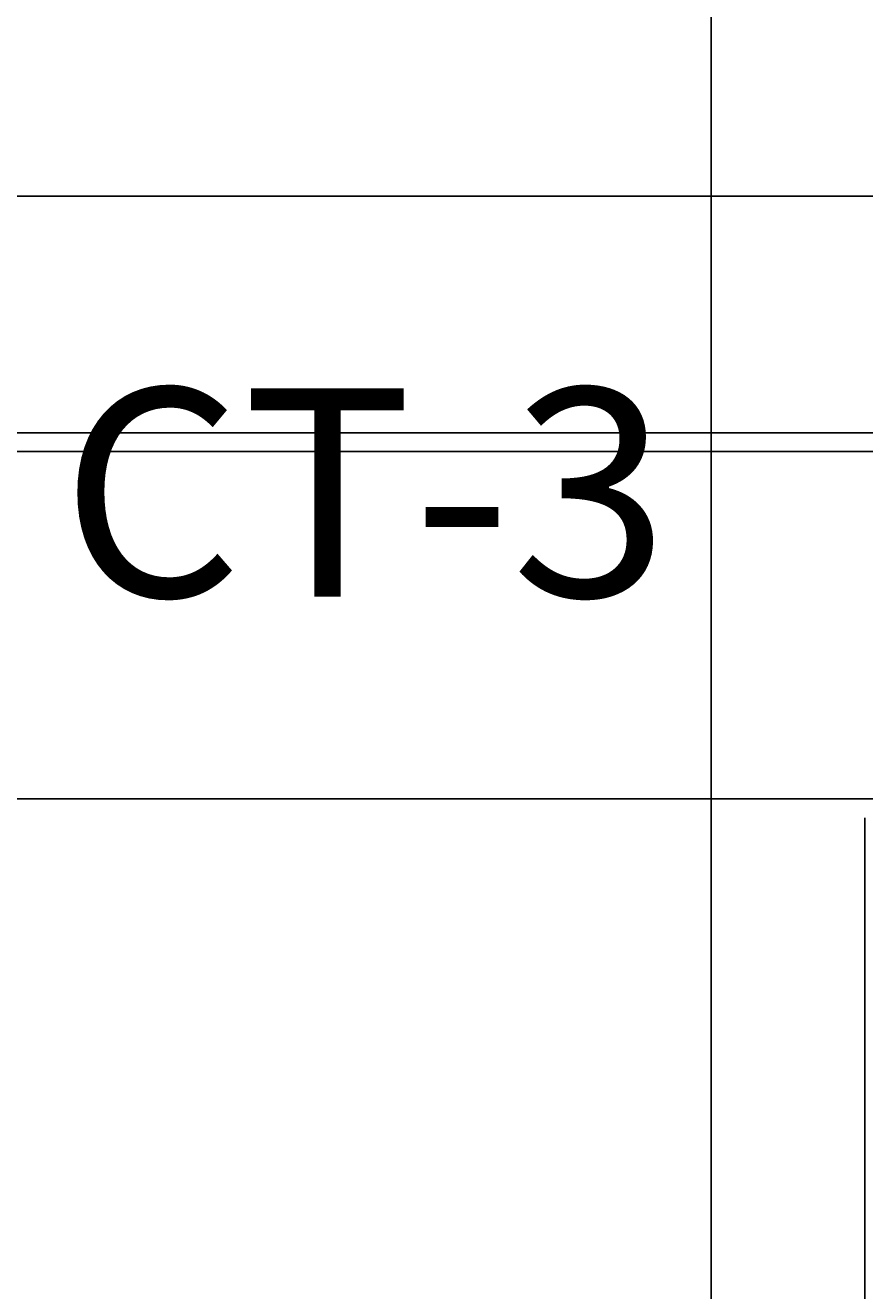
# Model space of a CAD drawing. Units: inches. Extents: x 35362 to 73946, y 43607 to 67532.
# Tile 133 of 134: x 67594 to 68484, y 44948 to 46290. Entities that reach past the tile are written whole.
import ezdxf

# ---------------------------------------------------------------- set-up
doc = ezdxf.new("R2010")
doc.units = ezdxf.units.IN
doc.header["$MEASUREMENT"] = 0
doc.layers.add('A-ANNO-DIMS', color=2, linetype='Continuous', lineweight=18)
doc.layers.add('E-ANNO-TEXT', color=5, linetype='Continuous', lineweight=18)
doc.styles.get("Standard").update_dxf_attribs({"font": 'arial.ttf'})
doc.dimstyles.get("Standard").update_dxf_attribs({"dimtxt": 0.18, "dimasz": 0.18, "dimexe": 0.18, "dimexo": 0.0625, "dimgap": 0.09, "dimtad": 0, "dimtih": 1, "dimtoh": 1, "dimdec": 4, "dimzin": 0, "dimdsep": 46, "dimtxsty": 'Standard', "dimcen": 0.09, "dimadec": 0, "dimazin": 0, "dimtfac": 1, "dimtdec": 4, "dimtofl": 0, "dimtmove": 0, "dimatfit": 3, "dimfxl": 1, "dimtolj": 1, "dimtzin": 0, "dimarcsym": 0})

# ---------------------------------------------------------------- blocks, each defined once
blk = doc.blocks.new('*D5')
at = {"layer": 'A-ANNO-DIMS', "color": 0, "lineweight": -2, "transparency": 16777216}
for p, q in [((37121.949085, 46919.318283), (37121.949085, 43606.678996)), ((69871.496302, 45449.831951), (69871.496302, 43606.678996)), ((37122.129085, 43606.858996), (53496.2943647142, 43606.858996)), ((69871.316302, 43606.858996), (53497.15102228581, 43606.858996))]:
    blk.add_line(p, q, dxfattribs=at)
at = {"layer": 'A-ANNO-DIMS', "color": 0, "transparency": 16777216}
for points in [[(37122.129085, 43606.888996), (37122.129085, 43606.828996), (37121.949085, 43606.858996)], [(69871.316302, 43606.888996), (69871.316302, 43606.828996), (69871.496302, 43606.858996)]]:
    blk.add_solid(points, dxfattribs=at)
at = {"layer": 'Defpoints', "color": 0, "transparency": 16777216}
for p in [(37121.949085, 46919.380783), (69871.496302, 45449.894451), (69871.496302, 43606.858996)]:
    blk.add_point(p, dxfattribs=at)
at = {"layer": 'A-ANNO-DIMS', "color": 0, "transparency": 16777216, "insert": (53496.7226935, 43606.858996), "char_height": 0.18, "attachment_point": 5}
blk.add_mtext('\\A1;32750', dxfattribs=at)
blk = doc.blocks.new('*D38')
at = {"layer": 'A-ANNO-DIMS', "color": 0, "lineweight": -2, "transparency": 16777216}
for p, q in [((68483.500128, 45449.831951), (68483.500128, 43606.678996)), ((62090.58505699999, 45366.796496), (62090.58505699999, 43606.678996)), ((62090.76505699999, 43606.858996), (65286.57828827081, 43606.858996)), ((68483.320128, 43606.858996), (65287.5068967292, 43606.858996))]:
    blk.add_line(p, q, dxfattribs=at)
at = {"layer": 'A-ANNO-DIMS', "color": 0, "transparency": 16777216}
for points in [[(62090.76505699999, 43606.888996), (62090.76505699999, 43606.828996), (62090.58505699999, 43606.858996)], [(68483.320128, 43606.888996), (68483.320128, 43606.828996), (68483.500128, 43606.858996)]]:
    blk.add_solid(points, dxfattribs=at)
at = {"layer": 'Defpoints', "color": 0, "transparency": 16777216}
for p in [(68483.500128, 45449.894451), (62090.58505699999, 45366.858996), (68483.500128, 43606.858996)]:
    blk.add_point(p, dxfattribs=at)
at = {"layer": 'A-ANNO-DIMS', "color": 0, "transparency": 16777216, "insert": (65287.0425925, 43606.858996), "char_height": 0.18, "attachment_point": 5}
blk.add_mtext('\\A1;6392.9', dxfattribs=at)
blk = doc.blocks.new('*D68')
at = {"layer": 'A-ANNO-DIMS', "color": 0, "lineweight": -2, "transparency": 16777216}
for p, q in [((68320.870762, 54372.885224), (68320.870762, 43606.678996)), ((61240.907336, 53351.466162), (61240.907336, 43606.678996)), ((61241.08733599999, 43606.858996), (64780.42646373397, 43606.858996)), ((68320.69076200001, 43606.858996), (64781.35163426603, 43606.858996))]:
    blk.add_line(p, q, dxfattribs=at)
at = {"layer": 'A-ANNO-DIMS', "color": 0, "transparency": 16777216}
for points in [[(61241.08733599999, 43606.888996), (61241.08733599999, 43606.828996), (61240.907336, 43606.858996)], [(68320.69076200001, 43606.888996), (68320.69076200001, 43606.828996), (68320.870762, 43606.858996)]]:
    blk.add_solid(points, dxfattribs=at)
at = {"layer": 'Defpoints', "color": 0, "transparency": 16777216}
for p in [(68320.870762, 54372.947724), (61240.907336, 53351.52866199999), (68320.870762, 43606.858996)]:
    blk.add_point(p, dxfattribs=at)
at = {"layer": 'A-ANNO-DIMS', "color": 0, "transparency": 16777216, "insert": (64780.889049, 43606.858996), "char_height": 0.18, "attachment_point": 5}
blk.add_mtext('\\A1;7080.0', dxfattribs=at)
blk = doc.blocks.new('*D74')
at = {"layer": 'A-ANNO-DIMS', "color": 0, "lineweight": -2, "transparency": 16777216}
for p, q in [((55181.69646300003, 46108.87757800001), (73945.82566600003, 46108.87757800001)), ((73945.64566600005, 46108.69757800001), (73945.64566600005, 45983.7251866378)), ((73945.64566600005, 45858.38898900001), (73945.64566600005, 45983.36138036223)), ((55181.69646300003, 45858.20898900001), (73945.82566600003, 45858.20898900001))]:
    blk.add_line(p, q, dxfattribs=at)
at = {"layer": 'A-ANNO-DIMS', "color": 0, "transparency": 16777216}
for points in [[(73945.61566600006, 46108.69757800001), (73945.67566600005, 46108.69757800001), (73945.64566600005, 46108.87757800001)], [(73945.61566600006, 45858.38898900001), (73945.67566600005, 45858.38898900001), (73945.64566600005, 45858.20898900001)]]:
    blk.add_solid(points, dxfattribs=at)
at = {"layer": 'Defpoints', "color": 0, "transparency": 16777216}
for p in [(55181.63396300002, 46108.87757800001), (55181.63396300002, 45858.20898900001), (73945.64566600005, 45858.20898900001)]:
    blk.add_point(p, dxfattribs=at)
at = {"layer": 'A-ANNO-DIMS', "color": 0, "transparency": 16777216, "insert": (73945.64566600005, 45983.54328349999), "char_height": 0.18, "attachment_point": 5}
blk.add_mtext('\\A1;250.67', dxfattribs=at)
blk = doc.blocks.new('*D75')
at = {"layer": 'A-ANNO-DIMS', "color": 0, "lineweight": -2, "transparency": 16777216}
for p, q in [((55181.69646300003, 45838.20898900001), (73945.82566600003, 45838.20898900001)), ((73945.64566600005, 45838.02898900001), (73945.64566600005, 45654.23368452933)), ((73945.64566600005, 45470.07445100001), (73945.64566600005, 45653.86975547068)), ((55181.69646300003, 45469.89445100001), (73945.82566600003, 45469.89445100001))]:
    blk.add_line(p, q, dxfattribs=at)
at = {"layer": 'A-ANNO-DIMS', "color": 0, "transparency": 16777216}
for points in [[(73945.61566600006, 45838.02898900001), (73945.67566600005, 45838.02898900001), (73945.64566600005, 45838.20898900001)], [(73945.61566600006, 45470.07445100001), (73945.67566600005, 45470.07445100001), (73945.64566600005, 45469.89445100001)]]:
    blk.add_solid(points, dxfattribs=at)
at = {"layer": 'Defpoints', "color": 0, "transparency": 16777216}
for p in [(55181.63396300002, 45838.20898900001), (55181.63396300002, 45469.89445100001), (73945.64566600005, 45469.89445100001)]:
    blk.add_point(p, dxfattribs=at)
at = {"layer": 'A-ANNO-DIMS', "color": 0, "transparency": 16777216, "insert": (73945.64566600005, 45654.05171999998), "char_height": 0.18, "attachment_point": 5}
blk.add_mtext('\\A1;368.3', dxfattribs=at)

msp = doc.modelspace()

# ---------------------------------------------------------------- texts
at = {"layer": 'E-ANNO-TEXT'}
msp.add_text('CT-3', height=220.8659825270206, dxfattribs=at).set_placement((67631.54899135625, 45684.41897833226))

# ---------------------------------------------------------------- dimensions: what is measured, and where the dimension line sits
at = {"layer": 'A-ANNO-DIMS'}
for base, p1, p2, override, picture, middle in [((68320.870762, 43606.858996), (61240.907336, 53351.52866199999), (68320.870762, 54372.947724), {"dimdec": 1, "dimlfac": 1, "dimrnd": 0, "dimzin": 0, "dimdsep": 46, "dimlunit": 2}, '*D68', (64780.889049, 43606.858996)), ((69871.496302, 43606.858996), (37121.949085, 46919.380783), (69871.496302, 45449.894451), {"dimdec": 0, "dimlfac": 1, "dimrnd": 0, "dimzin": 0, "dimdsep": 46, "dimlunit": 2}, '*D5', (53496.7226935, 43606.858996)), ((68483.500128, 43606.858996), (62090.58505699999, 45366.858996), (68483.500128, 45449.894451), {"dimdec": 1, "dimlfac": 1, "dimrnd": 0, "dimzin": 0, "dimdsep": 46, "dimlunit": 2}, '*D38', (65287.0425925, 43606.858996))]:
    dim = msp.add_linear_dim(base=base, p1=p1, p2=p2, dimstyle='Standard', override=override, dxfattribs=at)
    dim.commit()
    dim.dimension.update_dxf_attribs({"geometry": picture, "text_midpoint": middle})
for base, p1, p2, override, picture, middle in [((73945.64566600005, 45858.20898900001), (55181.633963, 46108.877578), (55181.633963, 45858.20898899999), {"dimdec": 2, "dimlfac": 1, "dimrnd": 0, "dimzin": 0, "dimdsep": 46, "dimlunit": 2}, '*D74', (73945.64566600005, 45983.54328349999)), ((73945.64566600005, 45469.89445100001), (55181.633963, 45838.20898899999), (55181.633963, 45469.894451), {"dimdec": 1, "dimlfac": 1, "dimrnd": 0, "dimzin": 0, "dimdsep": 46, "dimlunit": 2}, '*D75', (73945.64566600005, 45654.05171999998))]:
    dim = msp.add_linear_dim(base=base, p1=p1, p2=p2, angle=90, dimstyle='Standard', override=override, dxfattribs=at)
    dim.commit()
    dim.dimension.update_dxf_attribs({"geometry": picture, "text_midpoint": middle})

doc.saveas('drawing.dxf')
